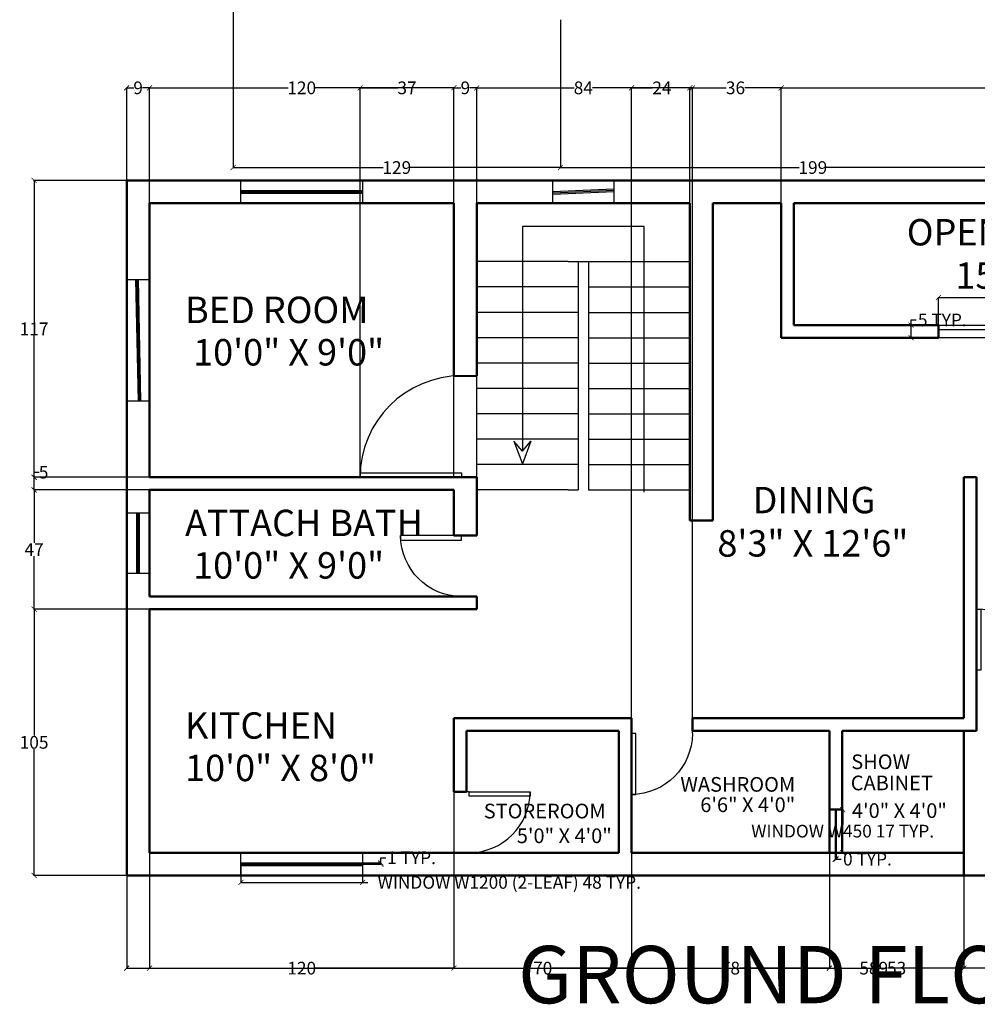
# Model space of a CAD drawing. Units: inches. Extents: x 1455 to 5994, y -182 to 2370.
# Tile 1 of 8: x 1509 to 1887, y 1415 to 1803. Entities that reach past the tile are written whole.
import ezdxf

# ---------------------------------------------------------------- set-up
doc = ezdxf.new("R2010")
doc.units = ezdxf.units.IN
doc.header["$MEASUREMENT"] = 0
for name, color, linetype, lineweight in [('A-ANNO-DIMS', 2, 'Continuous', 18), ('A-ANNO-TEXT', 7, 'Continuous', 25), ('A-AREA-IDEN', 7, 'Continuous', 18), ('A-DOOR', 5, 'Continuous', 25), ('A-FLOR-STRS', 3, 'Continuous', 25), ('A-GLAZ', 4, 'Continuous', 25), ('A-WALL', 7, 'Continuous', 50)]:
    doc.layers.add(name, color=color, linetype=linetype, lineweight=lineweight)
doc.styles.get("Standard").update_dxf_attribs({"font": 'arial.ttf'})
doc.dimstyles.get("Standard").update_dxf_attribs({"dimtxt": 5, "dimasz": 2, "dimexe": 0.18, "dimexo": 0.0625, "dimgap": 0.09, "dimtad": 0, "dimtih": 1, "dimtoh": 1, "dimdec": 1, "dimzin": 0, "dimdsep": 46, "dimlunit": 3, "dimtxsty": 'Standard', "dimblk": 'ARCHTICK', "dimcen": 0.09, "dimadec": 0, "dimazin": 0, "dimtfac": 1, "dimtdec": 1, "dimtofl": 0, "dimtmove": 0, "dimatfit": 3, "dimfxl": 1, "dimtolj": 1, "dimtzin": 0, "dimarcsym": 0})

# ---------------------------------------------------------------- blocks, each defined once
blk = doc.blocks.new('*U3')
for p, q in [((0, 0), (0, -6)), ((24, 0), (24, -6))]:
    blk.add_line(p, q)
blk.add_lwpolyline([(0, 0), (0, 24), (1.75, 24), (1.75, 0)], close=True)
blk.add_arc((0, 0), 24, 0, 90)
blk = doc.blocks.new('*U4')
for p, q in [((0, 0), (0, -6)), ((40, 0), (40, -6))]:
    blk.add_line(p, q)
blk.add_lwpolyline([(0, 0), (0, 40), (1.75, 40), (1.75, 0)], close=True)
blk.add_arc((0, 0), 40, 0, 90)
blk = doc.blocks.new('DOOR-SLIDING')
for p, q in [((37.51, 2.96), (37.51, 4.69)), ((0, 2.96), (37.51, 2.96)), ((34.07, 1.25), (34.07, 2.97)), ((72, 1.25), (34.07, 1.25)), ((37.51, 2.96), (72, 2.96))]:
    blk.add_line(p, q)
blk.add_lwpolyline([(0, 4.69), (72, 4.69), (72, -0.31), (0, -0.31)], close=True)
blk = doc.blocks.new('WIN-600')
for p, q in [((0, 0), (0, 24)), ((0.5, 0), (0.5, 24)), ((1, 0), (1, 24))]:
    blk.add_line(p, q)
blk = doc.blocks.new('WIN-1200')
for p, q in [((0, 1), (48, 1)), ((0, 0.5), (48, 0.5)), ((0, 0), (48, 0))]:
    blk.add_line(p, q)
blk = doc.blocks.new('WIN-1200-2L')
for p, q in [((0, 0.5), (48, 0.5)), ((0, 0), (48, 0))]:
    blk.add_line(p, q)
blk = doc.blocks.new('WIN-450')
for p, q in [((0, 17), (0, 0)), ((0.2, 17), (0.2, 0)), ((0.4, 17), (0.4, 0))]:
    blk.add_line(p, q)
blk = doc.blocks.new('_ArchTick')
at = {"color": 0, "linetype": 'ByBlock', "const_width": 0.15}
blk.add_lwpolyline([(-0.5, -0.5), (0.5, 0.5)], dxfattribs=at)
blk = doc.blocks.new('*D25')
at = {"layer": 'A-ANNO-DIMS', "color": 0, "lineweight": -2, "transparency": 16777216}
for p, q in [((1596.31, 1470.12), (1596.31, 1462.81)), ((1644.31, 1470.12), (1644.31, 1462.81)), ((1596.31, 1462.99), (1644.31, 1462.99)), ((1644.31, 1462.99), (1646.31, 1462.99))]:
    blk.add_line(p, q, dxfattribs=at)
at = {"layer": 'Defpoints', "color": 0, "lineweight": 25, "transparency": 16777216}
for p in [(1596.31, 1470.19), (1644.31, 1470.19), (1644.31, 1462.99)]:
    blk.add_point(p, dxfattribs=at)
at = {"layer": 'A-ANNO-DIMS', "color": 0, "lineweight": -2, "transparency": 16777216, "xscale": 2, "yscale": 2, "zscale": 2, "rotation": 180}
blk.add_blockref('_ArchTick', (1596.31, 1462.99), dxfattribs=at)
at = {"layer": 'A-ANNO-DIMS', "color": 0, "lineweight": -2, "transparency": 16777216, "xscale": 2, "yscale": 2, "zscale": 2}
blk.add_blockref('_ArchTick', (1644.31, 1462.99), dxfattribs=at)
at = {"layer": 'A-ANNO-DIMS', "color": 0, "transparency": 16777216, "insert": (1702.14, 1462.99), "char_height": 5, "attachment_point": 5}
blk.add_mtext('\\A1;WINDOW W1200 (2-LEAF) 48 TYP.', dxfattribs=at)
blk = doc.blocks.new('*D26')
at = {"layer": 'A-ANNO-DIMS', "color": 0, "lineweight": -2, "transparency": 16777216}
for p, q in [((1651.51, 1470.69), (1651.51, 1472.69)), ((1651.51, 1472.69), (1653.51, 1472.69)), ((1644.37, 1470.69), (1651.69, 1470.69)), ((1644.37, 1470.19), (1651.69, 1470.19)), ((1651.51, 1470.19), (1651.51, 1470.69))]:
    blk.add_line(p, q, dxfattribs=at)
at = {"layer": 'Defpoints', "color": 0, "lineweight": 25, "transparency": 16777216}
for p in [(1644.31, 1470.69), (1644.31, 1470.19), (1651.51, 1470.69)]:
    blk.add_point(p, dxfattribs=at)
at = {"layer": 'A-ANNO-DIMS', "color": 0, "lineweight": -2, "transparency": 16777216, "xscale": 2, "yscale": 2, "zscale": 2}
for p, rotation in [((1651.51, 1470.69), 90), ((1651.51, 1470.19), 270)]:
    blk.add_blockref('_ArchTick', p, dxfattribs=dict(at, rotation=rotation))
at = {"layer": 'A-ANNO-DIMS', "color": 0, "transparency": 16777216, "insert": (1663.59, 1472.69), "char_height": 5, "attachment_point": 5}
blk.add_mtext('\\A1;1 TYP.', dxfattribs=at)
blk = doc.blocks.new('*D27')
at = {"layer": 'A-ANNO-DIMS', "color": 0, "lineweight": -2, "transparency": 16777216}
for p, q in [((1831.07, 1491.69), (1833.74, 1491.69)), ((1833.56, 1491.69), (1833.56, 1485.86)), ((1833.56, 1474.69), (1833.56, 1480.51)), ((1831.07, 1474.69), (1833.74, 1474.69))]:
    blk.add_line(p, q, dxfattribs=at)
at = {"layer": 'Defpoints', "color": 0, "lineweight": 25, "transparency": 16777216}
for p in [(1831.01, 1491.69), (1833.56, 1491.69), (1831.01, 1474.69)]:
    blk.add_point(p, dxfattribs=at)
at = {"layer": 'A-ANNO-DIMS', "color": 0, "lineweight": -2, "transparency": 16777216, "xscale": 2, "yscale": 2, "zscale": 2}
for p, rotation in [((1833.56, 1491.69), 90), ((1833.56, 1474.69), 270)]:
    blk.add_blockref('_ArchTick', p, dxfattribs=dict(at, rotation=rotation))
at = {"layer": 'A-ANNO-DIMS', "color": 0, "transparency": 16777216, "insert": (1833.56, 1483.19), "char_height": 5, "attachment_point": 5}
blk.add_mtext('\\A1;WINDOW W450 17 TYP.', dxfattribs=at)
blk = doc.blocks.new('*D28')
at = {"layer": 'A-ANNO-DIMS', "color": 0, "lineweight": -2, "transparency": 16777216}
for p, q in [((1830.61, 1474.62), (1830.61, 1471.96)), ((1830.61, 1472.14), (1831.01, 1472.14)), ((1831.01, 1474.62), (1831.01, 1471.96)), ((1831.01, 1472.14), (1833.01, 1472.14))]:
    blk.add_line(p, q, dxfattribs=at)
at = {"layer": 'Defpoints', "color": 0, "lineweight": 25, "transparency": 16777216}
for p in [(1830.61, 1474.69), (1831.01, 1474.69), (1831.01, 1472.14)]:
    blk.add_point(p, dxfattribs=at)
at = {"layer": 'A-ANNO-DIMS', "color": 0, "lineweight": -2, "transparency": 16777216, "xscale": 2, "yscale": 2, "zscale": 2, "rotation": 180}
blk.add_blockref('_ArchTick', (1830.61, 1472.14), dxfattribs=at)
at = {"layer": 'A-ANNO-DIMS', "color": 0, "lineweight": -2, "transparency": 16777216, "xscale": 2, "yscale": 2, "zscale": 2}
blk.add_blockref('_ArchTick', (1831.01, 1472.14), dxfattribs=at)
at = {"layer": 'A-ANNO-DIMS', "color": 0, "transparency": 16777216, "insert": (1843.33, 1472.14), "char_height": 5, "attachment_point": 5}
blk.add_mtext('\\A1;0 TYP.', dxfattribs=at)
blk = doc.blocks.new('*D29')
at = {"layer": 'A-ANNO-DIMS', "color": 0, "lineweight": -2, "transparency": 16777216}
for p, q in [((1871.31, 1682.75), (1871.31, 1693.67)), ((1871.31, 1693.49), (1943.31, 1693.49)), ((1943.31, 1682.75), (1943.31, 1693.67)), ((1943.31, 1693.49), (1945.31, 1693.49))]:
    blk.add_line(p, q, dxfattribs=at)
at = {"layer": 'Defpoints', "color": 0, "lineweight": 25, "transparency": 16777216}
for p in [(1943.31, 1693.49), (1871.31, 1682.69), (1943.31, 1682.69)]:
    blk.add_point(p, dxfattribs=at)
at = {"layer": 'A-ANNO-DIMS', "color": 0, "lineweight": -2, "transparency": 16777216, "xscale": 2, "yscale": 2, "zscale": 2, "rotation": 180}
blk.add_blockref('_ArchTick', (1871.31, 1693.49), dxfattribs=at)
at = {"layer": 'A-ANNO-DIMS', "color": 0, "lineweight": -2, "transparency": 16777216, "xscale": 2, "yscale": 2, "zscale": 2}
blk.add_blockref('_ArchTick', (1943.31, 1693.49), dxfattribs=at)
at = {"layer": 'A-ANNO-DIMS', "color": 0, "transparency": 16777216, "insert": (1983.95, 1693.49), "char_height": 5, "attachment_point": 5}
blk.add_mtext('\\A1;SLIDING DOOR 72 TYP.', dxfattribs=at)
blk = doc.blocks.new('*D30')
at = {"layer": 'A-ANNO-DIMS', "color": 0, "lineweight": -2, "transparency": 16777216}
for p, q in [((1860.51, 1682.69), (1860.51, 1684.69)), ((1860.51, 1684.69), (1862.51, 1684.69)), ((1871.25, 1682.69), (1860.33, 1682.69)), ((1860.51, 1677.69), (1860.51, 1682.69)), ((1871.25, 1677.69), (1860.33, 1677.69))]:
    blk.add_line(p, q, dxfattribs=at)
at = {"layer": 'Defpoints', "color": 0, "lineweight": 25, "transparency": 16777216}
for p in [(1860.51, 1682.69), (1871.31, 1682.69), (1871.31, 1677.69)]:
    blk.add_point(p, dxfattribs=at)
at = {"layer": 'A-ANNO-DIMS', "color": 0, "lineweight": -2, "transparency": 16777216, "xscale": 2, "yscale": 2, "zscale": 2}
for p, rotation in [((1860.51, 1682.69), 90), ((1860.51, 1677.69), 270)]:
    blk.add_blockref('_ArchTick', p, dxfattribs=dict(at, rotation=rotation))
at = {"layer": 'A-ANNO-DIMS', "color": 0, "transparency": 16777216, "insert": (1872.83, 1684.69), "char_height": 5, "attachment_point": 5}
blk.add_mtext('\\A1;5 TYP.', dxfattribs=at)
blk = doc.blocks.new('*D35')
at = {"layer": 'A-ANNO-DIMS', "color": 0, "lineweight": -2, "transparency": 16777216}
for p, q in [((1593.29, 1828.67), (1593.29, 1744.59)), ((1722.29, 1802.99), (1722.29, 1744.59)), ((1593.29, 1744.77), (1652.41, 1744.77)), ((1722.29, 1744.77), (1663.18, 1744.77))]:
    blk.add_line(p, q, dxfattribs=at)
at = {"layer": 'Defpoints', "color": 0, "lineweight": 25, "transparency": 16777216}
for p in [(1593.29, 1828.73), (1722.29, 1803.05), (1722.29, 1744.77)]:
    blk.add_point(p, dxfattribs=at)
at = {"layer": 'A-ANNO-DIMS', "color": 0, "lineweight": -2, "transparency": 16777216, "xscale": 2, "yscale": 2, "zscale": 2, "rotation": 180}
blk.add_blockref('_ArchTick', (1593.29, 1744.77), dxfattribs=at)
at = {"layer": 'A-ANNO-DIMS', "color": 0, "lineweight": -2, "transparency": 16777216, "xscale": 2, "yscale": 2, "zscale": 2}
blk.add_blockref('_ArchTick', (1722.29, 1744.77), dxfattribs=at)
at = {"layer": 'A-ANNO-DIMS', "color": 0, "transparency": 16777216, "insert": (1657.79, 1744.77), "char_height": 5, "attachment_point": 5}
blk.add_mtext('\\A1;129', dxfattribs=at)
blk = doc.blocks.new('*D36')
at = {"layer": 'A-ANNO-DIMS', "color": 0, "lineweight": -2, "transparency": 16777216}
for p, q in [((1722.29, 1802.99), (1722.29, 1744.59)), ((1921.29, 1801.67), (1921.29, 1744.59)), ((1722.29, 1744.77), (1816.41, 1744.77)), ((1921.29, 1744.77), (1827.18, 1744.77))]:
    blk.add_line(p, q, dxfattribs=at)
at = {"layer": 'Defpoints', "color": 0, "lineweight": 25, "transparency": 16777216}
for p in [(1722.29, 1803.05), (1921.29, 1801.73), (1921.29, 1744.77)]:
    blk.add_point(p, dxfattribs=at)
at = {"layer": 'A-ANNO-DIMS', "color": 0, "lineweight": -2, "transparency": 16777216, "xscale": 2, "yscale": 2, "zscale": 2, "rotation": 180}
blk.add_blockref('_ArchTick', (1722.29, 1744.77), dxfattribs=at)
at = {"layer": 'A-ANNO-DIMS', "color": 0, "lineweight": -2, "transparency": 16777216, "xscale": 2, "yscale": 2, "zscale": 2}
blk.add_blockref('_ArchTick', (1921.29, 1744.77), dxfattribs=at)
at = {"layer": 'A-ANNO-DIMS', "color": 0, "transparency": 16777216, "insert": (1821.79, 1744.77), "char_height": 5, "attachment_point": 5}
blk.add_mtext('\\A1;199', dxfattribs=at)
blk = doc.blocks.new('*D43')
at = {"layer": 'A-ANNO-DIMS', "color": 0, "lineweight": -2, "transparency": 16777216}
for p, q in [((1551.31, 1465.62), (1551.31, 1429.01)), ((2140.31, 1465.62), (2140.31, 1429.01)), ((1551.31, 1429.19), (1840.19, 1429.19)), ((2140.31, 1429.19), (1851.43, 1429.19))]:
    blk.add_line(p, q, dxfattribs=at)
at = {"layer": 'Defpoints', "color": 0, "lineweight": 25, "transparency": 16777216}
for p in [(1551.31, 1465.69), (2140.31, 1465.69), (2140.31, 1429.19)]:
    blk.add_point(p, dxfattribs=at)
at = {"layer": 'A-ANNO-DIMS', "color": 0, "lineweight": -2, "transparency": 16777216, "xscale": 2, "yscale": 2, "zscale": 2, "rotation": 180}
blk.add_blockref('_ArchTick', (1551.31, 1429.19), dxfattribs=at)
at = {"layer": 'A-ANNO-DIMS', "color": 0, "lineweight": -2, "transparency": 16777216, "xscale": 2, "yscale": 2, "zscale": 2}
blk.add_blockref('_ArchTick', (2140.31, 1429.19), dxfattribs=at)
at = {"layer": 'A-ANNO-DIMS', "color": 0, "transparency": 16777216, "insert": (1845.81, 1429.19), "char_height": 5, "attachment_point": 5}
blk.add_mtext('\\A1;589', dxfattribs=at)
blk = doc.blocks.new('*D45')
at = {"layer": 'A-ANNO-DIMS', "color": 0, "lineweight": -2, "transparency": 16777216}
for p, q in [((1551.31, 1739.75), (1551.31, 1776.37)), ((1551.31, 1776.19), (1554.08, 1776.19)), ((1560.31, 1776.19), (1557.55, 1776.19)), ((1560.31, 1700.75), (1560.31, 1776.37))]:
    blk.add_line(p, q, dxfattribs=at)
at = {"layer": 'Defpoints', "color": 0, "lineweight": 25, "transparency": 16777216}
for p in [(1560.31, 1776.19), (1551.31, 1739.69), (1560.31, 1700.69)]:
    blk.add_point(p, dxfattribs=at)
at = {"layer": 'A-ANNO-DIMS', "color": 0, "lineweight": -2, "transparency": 16777216, "xscale": 2, "yscale": 2, "zscale": 2, "rotation": 180}
blk.add_blockref('_ArchTick', (1551.31, 1776.19), dxfattribs=at)
at = {"layer": 'A-ANNO-DIMS', "color": 0, "lineweight": -2, "transparency": 16777216, "xscale": 2, "yscale": 2, "zscale": 2}
blk.add_blockref('_ArchTick', (1560.31, 1776.19), dxfattribs=at)
at = {"layer": 'A-ANNO-DIMS', "color": 0, "transparency": 16777216, "insert": (1555.81, 1776.19), "char_height": 5, "attachment_point": 5}
blk.add_mtext('\\A1;9', dxfattribs=at)
blk = doc.blocks.new('*D46')
at = {"layer": 'A-ANNO-DIMS', "color": 0, "lineweight": -2, "transparency": 16777216}
for p, q in [((1560.31, 1700.75), (1560.31, 1776.37)), ((1560.31, 1776.19), (1614.94, 1776.19)), ((1680.31, 1776.19), (1625.68, 1776.19)), ((1680.31, 1730.75), (1680.31, 1776.37))]:
    blk.add_line(p, q, dxfattribs=at)
at = {"layer": 'Defpoints', "color": 0, "lineweight": 25, "transparency": 16777216}
for p in [(1680.31, 1776.19), (1680.31, 1730.69), (1560.31, 1700.69)]:
    blk.add_point(p, dxfattribs=at)
at = {"layer": 'A-ANNO-DIMS', "color": 0, "lineweight": -2, "transparency": 16777216, "xscale": 2, "yscale": 2, "zscale": 2, "rotation": 180}
blk.add_blockref('_ArchTick', (1560.31, 1776.19), dxfattribs=at)
at = {"layer": 'A-ANNO-DIMS', "color": 0, "lineweight": -2, "transparency": 16777216, "xscale": 2, "yscale": 2, "zscale": 2}
blk.add_blockref('_ArchTick', (1680.31, 1776.19), dxfattribs=at)
at = {"layer": 'A-ANNO-DIMS', "color": 0, "transparency": 16777216, "insert": (1620.31, 1776.19), "char_height": 5, "attachment_point": 5}
blk.add_mtext('\\A1;120', dxfattribs=at)
blk = doc.blocks.new('*D47')
at = {"layer": 'A-ANNO-DIMS', "color": 0, "lineweight": -2, "transparency": 16777216}
for p, q in [((1680.31, 1730.75), (1680.31, 1776.37)), ((1680.31, 1776.19), (1683.08, 1776.19)), ((1689.31, 1776.19), (1686.55, 1776.19)), ((1689.31, 1730.75), (1689.31, 1776.37))]:
    blk.add_line(p, q, dxfattribs=at)
at = {"layer": 'Defpoints', "color": 0, "lineweight": 25, "transparency": 16777216}
for p in [(1689.31, 1776.19), (1680.31, 1730.69), (1689.31, 1730.69)]:
    blk.add_point(p, dxfattribs=at)
at = {"layer": 'A-ANNO-DIMS', "color": 0, "lineweight": -2, "transparency": 16777216, "xscale": 2, "yscale": 2, "zscale": 2, "rotation": 180}
blk.add_blockref('_ArchTick', (1680.31, 1776.19), dxfattribs=at)
at = {"layer": 'A-ANNO-DIMS', "color": 0, "lineweight": -2, "transparency": 16777216, "xscale": 2, "yscale": 2, "zscale": 2}
blk.add_blockref('_ArchTick', (1689.31, 1776.19), dxfattribs=at)
at = {"layer": 'A-ANNO-DIMS', "color": 0, "transparency": 16777216, "insert": (1684.81, 1776.19), "char_height": 5, "attachment_point": 5}
blk.add_mtext('\\A1;9', dxfattribs=at)
blk = doc.blocks.new('*D48')
at = {"layer": 'A-ANNO-DIMS', "color": 0, "lineweight": -2, "transparency": 16777216}
for p, q in [((1689.31, 1730.75), (1689.31, 1776.37)), ((1689.31, 1776.19), (1727.65, 1776.19)), ((1773.31, 1776.19), (1734.98, 1776.19)), ((1773.31, 1730.75), (1773.31, 1776.37))]:
    blk.add_line(p, q, dxfattribs=at)
at = {"layer": 'Defpoints', "color": 0, "lineweight": 25, "transparency": 16777216}
for p in [(1773.31, 1776.19), (1689.31, 1730.69), (1773.31, 1730.69)]:
    blk.add_point(p, dxfattribs=at)
at = {"layer": 'A-ANNO-DIMS', "color": 0, "lineweight": -2, "transparency": 16777216, "xscale": 2, "yscale": 2, "zscale": 2, "rotation": 180}
blk.add_blockref('_ArchTick', (1689.31, 1776.19), dxfattribs=at)
at = {"layer": 'A-ANNO-DIMS', "color": 0, "lineweight": -2, "transparency": 16777216, "xscale": 2, "yscale": 2, "zscale": 2}
blk.add_blockref('_ArchTick', (1773.31, 1776.19), dxfattribs=at)
at = {"layer": 'A-ANNO-DIMS', "color": 0, "transparency": 16777216, "insert": (1731.31, 1776.19), "char_height": 5, "attachment_point": 5}
blk.add_mtext('\\A1;84', dxfattribs=at)
blk = doc.blocks.new('*D49')
at = {"layer": 'A-ANNO-DIMS', "color": 0, "lineweight": -2, "transparency": 16777216}
for p, q in [((1773.31, 1730.75), (1773.31, 1776.37)), ((1773.31, 1776.19), (1787.64, 1776.19)), ((1809.31, 1776.19), (1794.98, 1776.19)), ((1809.31, 1730.75), (1809.31, 1776.37))]:
    blk.add_line(p, q, dxfattribs=at)
at = {"layer": 'Defpoints', "color": 0, "lineweight": 25, "transparency": 16777216}
for p in [(1809.31, 1776.19), (1773.31, 1730.69), (1809.31, 1730.69)]:
    blk.add_point(p, dxfattribs=at)
at = {"layer": 'A-ANNO-DIMS', "color": 0, "lineweight": -2, "transparency": 16777216, "xscale": 2, "yscale": 2, "zscale": 2, "rotation": 180}
blk.add_blockref('_ArchTick', (1773.31, 1776.19), dxfattribs=at)
at = {"layer": 'A-ANNO-DIMS', "color": 0, "lineweight": -2, "transparency": 16777216, "xscale": 2, "yscale": 2, "zscale": 2}
blk.add_blockref('_ArchTick', (1809.31, 1776.19), dxfattribs=at)
at = {"layer": 'A-ANNO-DIMS', "color": 0, "transparency": 16777216, "insert": (1791.31, 1776.19), "char_height": 5, "attachment_point": 5}
blk.add_mtext('\\A1;36', dxfattribs=at)
blk = doc.blocks.new('*D50')
at = {"layer": 'A-ANNO-DIMS', "color": 0, "lineweight": -2, "transparency": 16777216}
for p, q in [((1809.31, 1730.75), (1809.31, 1776.37)), ((1809.31, 1776.19), (1901.94, 1776.19)), ((2005.31, 1776.19), (1912.69, 1776.19)), ((2005.31, 1730.75), (2005.31, 1776.37))]:
    blk.add_line(p, q, dxfattribs=at)
at = {"layer": 'Defpoints', "color": 0, "lineweight": 25, "transparency": 16777216}
for p in [(2005.31, 1776.19), (1809.31, 1730.69), (2005.31, 1730.69)]:
    blk.add_point(p, dxfattribs=at)
at = {"layer": 'A-ANNO-DIMS', "color": 0, "lineweight": -2, "transparency": 16777216, "xscale": 2, "yscale": 2, "zscale": 2, "rotation": 180}
blk.add_blockref('_ArchTick', (1809.31, 1776.19), dxfattribs=at)
at = {"layer": 'A-ANNO-DIMS', "color": 0, "lineweight": -2, "transparency": 16777216, "xscale": 2, "yscale": 2, "zscale": 2}
blk.add_blockref('_ArchTick', (2005.31, 1776.19), dxfattribs=at)
at = {"layer": 'A-ANNO-DIMS', "color": 0, "transparency": 16777216, "insert": (1907.31, 1776.19), "char_height": 5, "attachment_point": 5}
blk.add_mtext('\\A1;196', dxfattribs=at)
blk = doc.blocks.new('*D53')
at = {"layer": 'A-ANNO-DIMS', "color": 0, "lineweight": -2, "transparency": 16777216}
for p, q in [((1560.25, 1570.69), (1514.63, 1570.69)), ((1514.81, 1570.69), (1514.81, 1520.83)), ((1514.81, 1465.69), (1514.81, 1515.54)), ((2140.25, 1465.69), (1514.63, 1465.69))]:
    blk.add_line(p, q, dxfattribs=at)
at = {"layer": 'Defpoints', "color": 0, "lineweight": 25, "transparency": 16777216}
for p in [(1514.81, 1570.69), (1560.31, 1570.69), (2140.31, 1465.69)]:
    blk.add_point(p, dxfattribs=at)
at = {"layer": 'A-ANNO-DIMS', "color": 0, "lineweight": -2, "transparency": 16777216, "xscale": 2, "yscale": 2, "zscale": 2}
for p, rotation in [((1514.81, 1570.69), 90), ((1514.81, 1465.69), 270)]:
    blk.add_blockref('_ArchTick', p, dxfattribs=dict(at, rotation=rotation))
at = {"layer": 'A-ANNO-DIMS', "color": 0, "transparency": 16777216, "insert": (1514.81, 1518.19), "char_height": 5, "attachment_point": 5}
blk.add_mtext('\\A1;105', dxfattribs=at)
blk = doc.blocks.new('*D54')
at = {"layer": 'A-ANNO-DIMS', "color": 0, "lineweight": -2, "transparency": 16777216}
for p, q in [((1560.249038, 1617.686089), (1514.631538, 1617.686089)), ((1514.811538, 1617.686089), (1514.811538, 1596.776089)), ((1514.811538, 1570.686089), (1514.811538, 1591.596089)), ((1560.249038, 1570.686089), (1514.631538, 1570.686089))]:
    blk.add_line(p, q, dxfattribs=at)
at = {"layer": 'Defpoints', "color": 0, "lineweight": 25, "transparency": 16777216}
for p in [(1514.811538, 1617.686089), (1560.311538, 1617.686089), (1560.311538, 1570.686089)]:
    blk.add_point(p, dxfattribs=at)
at = {"layer": 'A-ANNO-DIMS', "color": 0, "lineweight": -2, "transparency": 16777216, "xscale": 2, "yscale": 2, "zscale": 2}
for p, rotation in [((1514.811538, 1617.686089), 90), ((1514.811538, 1570.686089), 270)]:
    blk.add_blockref('_ArchTick', p, dxfattribs=dict(at, rotation=rotation))
at = {"layer": 'A-ANNO-DIMS', "color": 0, "transparency": 16777216, "insert": (1514.811538, 1594.186089), "char_height": 5, "attachment_point": 5}
blk.add_mtext('\\A1;47', dxfattribs=at)
blk = doc.blocks.new('*D55')
at = {"layer": 'A-ANNO-DIMS', "color": 0, "lineweight": -2, "transparency": 16777216}
for p, q in [((1560.25, 1622.69), (1514.63, 1622.69)), ((1514.81, 1622.69), (1514.81, 1624.69)), ((1514.81, 1624.69), (1516.81, 1624.69)), ((1514.81, 1617.69), (1514.81, 1622.69)), ((1560.25, 1617.69), (1514.63, 1617.69))]:
    blk.add_line(p, q, dxfattribs=at)
at = {"layer": 'Defpoints', "color": 0, "lineweight": 25, "transparency": 16777216}
for p in [(1514.81, 1622.69), (1560.31, 1622.69), (1560.31, 1617.69)]:
    blk.add_point(p, dxfattribs=at)
at = {"layer": 'A-ANNO-DIMS', "color": 0, "lineweight": -2, "transparency": 16777216, "xscale": 2, "yscale": 2, "zscale": 2}
for p, rotation in [((1514.81, 1622.69), 90), ((1514.81, 1617.69), 270)]:
    blk.add_blockref('_ArchTick', p, dxfattribs=dict(at, rotation=rotation))
at = {"layer": 'A-ANNO-DIMS', "color": 0, "transparency": 16777216, "insert": (1518.56, 1624.69), "char_height": 5, "attachment_point": 5}
blk.add_mtext('\\A1;5', dxfattribs=at)
blk = doc.blocks.new('*D56')
at = {"layer": 'A-ANNO-DIMS', "color": 0, "lineweight": -2, "transparency": 16777216}
for p, q in [((1551.25, 1739.69), (1514.63, 1739.69)), ((1514.81, 1739.69), (1514.81, 1683.79)), ((1514.81, 1622.69), (1514.81, 1678.59)), ((1560.25, 1622.69), (1514.63, 1622.69))]:
    blk.add_line(p, q, dxfattribs=at)
at = {"layer": 'Defpoints', "color": 0, "lineweight": 25, "transparency": 16777216}
for p in [(1514.81, 1739.69), (1551.31, 1739.69), (1560.31, 1622.69)]:
    blk.add_point(p, dxfattribs=at)
at = {"layer": 'A-ANNO-DIMS', "color": 0, "lineweight": -2, "transparency": 16777216, "xscale": 2, "yscale": 2, "zscale": 2}
for p, rotation in [((1514.81, 1739.69), 90), ((1514.81, 1622.69), 270)]:
    blk.add_blockref('_ArchTick', p, dxfattribs=dict(at, rotation=rotation))
at = {"layer": 'A-ANNO-DIMS', "color": 0, "transparency": 16777216, "insert": (1514.81, 1681.19), "char_height": 5, "attachment_point": 5}
blk.add_mtext('\\A1;117', dxfattribs=at)
blk = doc.blocks.new('*D60')
at = {"layer": 'A-ANNO-DIMS', "color": 0, "lineweight": -2, "transparency": 16777216}
for p, q in [((1643.31, 1622.75), (1643.31, 1776.37)), ((1643.31, 1776.19), (1658.14, 1776.19)), ((1680.31, 1776.19), (1665.48, 1776.19)), ((1680.31, 1622.75), (1680.31, 1776.37))]:
    blk.add_line(p, q, dxfattribs=at)
at = {"layer": 'Defpoints', "color": 0, "lineweight": 25, "transparency": 16777216}
for p in [(1680.31, 1776.19), (1643.31, 1622.69), (1680.31, 1622.69)]:
    blk.add_point(p, dxfattribs=at)
at = {"layer": 'A-ANNO-DIMS', "color": 0, "lineweight": -2, "transparency": 16777216, "xscale": 2, "yscale": 2, "zscale": 2, "rotation": 180}
blk.add_blockref('_ArchTick', (1643.31, 1776.19), dxfattribs=at)
at = {"layer": 'A-ANNO-DIMS', "color": 0, "lineweight": -2, "transparency": 16777216, "xscale": 2, "yscale": 2, "zscale": 2}
blk.add_blockref('_ArchTick', (1680.31, 1776.19), dxfattribs=at)
at = {"layer": 'A-ANNO-DIMS', "color": 0, "transparency": 16777216, "insert": (1661.81, 1776.19), "char_height": 5, "attachment_point": 5}
blk.add_mtext('\\A1;37', dxfattribs=at)
blk = doc.blocks.new('*D63')
at = {"layer": 'A-ANNO-DIMS', "color": 0, "lineweight": -2, "transparency": 16777216}
for p, q in [((1680.31, 1498.62), (1680.31, 1429.01)), ((1560.31, 1474.62), (1560.31, 1429.01)), ((1560.31, 1429.19), (1614.94, 1429.19)), ((1680.31, 1429.19), (1625.68, 1429.19))]:
    blk.add_line(p, q, dxfattribs=at)
at = {"layer": 'Defpoints', "color": 0, "lineweight": 25, "transparency": 16777216}
for p in [(1680.31, 1498.69), (1560.31, 1474.69), (1680.31, 1429.19)]:
    blk.add_point(p, dxfattribs=at)
at = {"layer": 'A-ANNO-DIMS', "color": 0, "lineweight": -2, "transparency": 16777216, "xscale": 2, "yscale": 2, "zscale": 2, "rotation": 180}
blk.add_blockref('_ArchTick', (1560.31, 1429.19), dxfattribs=at)
at = {"layer": 'A-ANNO-DIMS', "color": 0, "lineweight": -2, "transparency": 16777216, "xscale": 2, "yscale": 2, "zscale": 2}
blk.add_blockref('_ArchTick', (1680.31, 1429.19), dxfattribs=at)
at = {"layer": 'A-ANNO-DIMS', "color": 0, "transparency": 16777216, "insert": (1620.31, 1429.19), "char_height": 5, "attachment_point": 5}
blk.add_mtext('\\A1;120', dxfattribs=at)
blk = doc.blocks.new('*D64')
at = {"layer": 'A-ANNO-DIMS', "color": 0, "lineweight": -2, "transparency": 16777216}
for p, q in [((1680.31, 1498.62), (1680.31, 1429.01)), ((1750.31, 1474.62), (1750.31, 1429.01)), ((1680.31, 1429.19), (1711.67, 1429.19)), ((1750.31, 1429.19), (1718.95, 1429.19))]:
    blk.add_line(p, q, dxfattribs=at)
at = {"layer": 'Defpoints', "color": 0, "lineweight": 25, "transparency": 16777216}
for p in [(1680.31, 1498.69), (1750.31, 1474.69), (1750.31, 1429.19)]:
    blk.add_point(p, dxfattribs=at)
at = {"layer": 'A-ANNO-DIMS', "color": 0, "lineweight": -2, "transparency": 16777216, "xscale": 2, "yscale": 2, "zscale": 2, "rotation": 180}
blk.add_blockref('_ArchTick', (1680.31, 1429.19), dxfattribs=at)
at = {"layer": 'A-ANNO-DIMS', "color": 0, "lineweight": -2, "transparency": 16777216, "xscale": 2, "yscale": 2, "zscale": 2}
blk.add_blockref('_ArchTick', (1750.31, 1429.19), dxfattribs=at)
at = {"layer": 'A-ANNO-DIMS', "color": 0, "transparency": 16777216, "insert": (1715.31, 1429.19), "char_height": 5, "attachment_point": 5}
blk.add_mtext('\\A1;70', dxfattribs=at)
blk = doc.blocks.new('*D65')
at = {"layer": 'A-ANNO-DIMS', "color": 0, "lineweight": -2, "transparency": 16777216}
for p, q in [((1750.31, 1474.62), (1750.31, 1429.01)), ((1828.31, 1474.62), (1828.31, 1429.01)), ((1750.31, 1429.19), (1785.66, 1429.19)), ((1828.31, 1429.19), (1792.97, 1429.19))]:
    blk.add_line(p, q, dxfattribs=at)
at = {"layer": 'Defpoints', "color": 0, "lineweight": 25, "transparency": 16777216}
for p in [(1750.31, 1474.69), (1828.31, 1474.69), (1828.31, 1429.19)]:
    blk.add_point(p, dxfattribs=at)
at = {"layer": 'A-ANNO-DIMS', "color": 0, "lineweight": -2, "transparency": 16777216, "xscale": 2, "yscale": 2, "zscale": 2, "rotation": 180}
blk.add_blockref('_ArchTick', (1750.31, 1429.19), dxfattribs=at)
at = {"layer": 'A-ANNO-DIMS', "color": 0, "lineweight": -2, "transparency": 16777216, "xscale": 2, "yscale": 2, "zscale": 2}
blk.add_blockref('_ArchTick', (1828.31, 1429.19), dxfattribs=at)
at = {"layer": 'A-ANNO-DIMS', "color": 0, "transparency": 16777216, "insert": (1789.31, 1429.19), "char_height": 5, "attachment_point": 5}
blk.add_mtext('\\A1;78', dxfattribs=at)
blk = doc.blocks.new('*D66')
at = {"layer": 'A-ANNO-DIMS', "color": 0, "lineweight": -2, "transparency": 16777216}
for p, q in [((1828.31, 1474.62), (1828.31, 1429.01)), ((1881.31, 1474.62), (1881.31, 1429.01)), ((1828.31, 1429.19), (1851.14, 1429.19)), ((1881.31, 1429.19), (1858.48, 1429.19))]:
    blk.add_line(p, q, dxfattribs=at)
at = {"layer": 'Defpoints', "color": 0, "lineweight": 25, "transparency": 16777216}
for p in [(1828.31, 1474.69), (1881.31, 1474.69), (1881.31, 1429.19)]:
    blk.add_point(p, dxfattribs=at)
at = {"layer": 'A-ANNO-DIMS', "color": 0, "lineweight": -2, "transparency": 16777216, "xscale": 2, "yscale": 2, "zscale": 2, "rotation": 180}
blk.add_blockref('_ArchTick', (1828.31, 1429.19), dxfattribs=at)
at = {"layer": 'A-ANNO-DIMS', "color": 0, "lineweight": -2, "transparency": 16777216, "xscale": 2, "yscale": 2, "zscale": 2}
blk.add_blockref('_ArchTick', (1881.31, 1429.19), dxfattribs=at)
at = {"layer": 'A-ANNO-DIMS', "color": 0, "transparency": 16777216, "insert": (1854.81, 1429.19), "char_height": 5, "attachment_point": 5}
blk.add_mtext('\\A1;53', dxfattribs=at)
blk = doc.blocks.new('*D67')
at = {"layer": 'A-ANNO-DIMS', "color": 0, "lineweight": -2, "transparency": 16777216}
for p, q in [((1750.31, 1527.75), (1750.31, 1776.37)), ((1750.31, 1776.19), (1758.61, 1776.19)), ((1774.31, 1776.19), (1766.02, 1776.19)), ((1774.31, 1527.75), (1774.31, 1776.37))]:
    blk.add_line(p, q, dxfattribs=at)
at = {"layer": 'Defpoints', "color": 0, "lineweight": 25, "transparency": 16777216}
for p in [(1774.31, 1776.19), (1750.31, 1527.69), (1774.31, 1527.69)]:
    blk.add_point(p, dxfattribs=at)
at = {"layer": 'A-ANNO-DIMS', "color": 0, "lineweight": -2, "transparency": 16777216, "xscale": 2, "yscale": 2, "zscale": 2, "rotation": 180}
blk.add_blockref('_ArchTick', (1750.31, 1776.19), dxfattribs=at)
at = {"layer": 'A-ANNO-DIMS', "color": 0, "lineweight": -2, "transparency": 16777216, "xscale": 2, "yscale": 2, "zscale": 2}
blk.add_blockref('_ArchTick', (1774.31, 1776.19), dxfattribs=at)
at = {"layer": 'A-ANNO-DIMS', "color": 0, "transparency": 16777216, "insert": (1762.31, 1776.19), "char_height": 5, "attachment_point": 5}
blk.add_mtext('\\A1;24', dxfattribs=at)

msp = doc.modelspace()

# ---------------------------------------------------------------- linework, layer by layer
at = {"layer": 'A-FLOR-STRS'}
for p, q in [((1755.3115, 1721.5573), (1707.3115, 1721.5573)), ((1707.3115, 1721.5573), (1707.3115, 1632.9997)), ((1755.3115, 1616.8618), (1755.3115, 1721.5573)), ((1725.3115, 1707.6861), (1689.3115, 1707.6861)), ((1725.3115, 1707.6861), (1737.3115, 1707.6861)), ((1729.3115, 1707.6861), (1729.3115, 1617.6861)), ((1733.3115, 1707.6861), (1733.3115, 1617.6861)), ((1737.3115, 1707.6861), (1773.3115, 1707.6861)), ((1729.3115, 1697.6861), (1689.3115, 1697.6861)), ((1733.3115, 1697.6861), (1773.3115, 1697.6861)), ((1729.3115, 1687.6861), (1689.3115, 1687.6861)), ((1733.3115, 1687.6861), (1773.3115, 1687.6861)), ((1729.3115, 1677.6861), (1689.3115, 1677.6861)), ((1733.3115, 1677.6861), (1773.3115, 1677.6861)), ((1729.3115, 1667.6861), (1689.3115, 1667.6861)), ((1733.3115, 1667.6861), (1773.3115, 1667.6861)), ((1689.3115, 1617.6861), (1689.3115, 1664.6861)), ((1729.3115, 1657.6861), (1689.3115, 1657.6861)), ((1733.3115, 1657.6861), (1773.3115, 1657.6861)), ((1729.3115, 1647.6861), (1689.3115, 1647.6861)), ((1733.3115, 1647.6861), (1773.3115, 1647.6861)), ((1729.3115, 1637.6861), (1689.3115, 1637.6861)), ((1707.3115, 1632.9997), (1703.9639, 1636.8618)), ((1703.9639, 1636.8618), (1707.3115, 1627.9809)), ((1707.3115, 1632.9997), (1710.6592, 1636.8618)), ((1710.6592, 1636.8618), (1707.3115, 1627.9809)), ((1733.3115, 1637.6861), (1773.3115, 1637.6861)), ((1729.3115, 1627.6861), (1689.3115, 1627.6861)), ((1733.3115, 1627.6861), (1773.3115, 1627.6861)), ((1725.3115, 1617.6861), (1689.3115, 1617.6861)), ((1725.3115, 1617.6861), (1729.3115, 1617.6861)), ((1733.3115, 1617.6861), (1737.3115, 1617.6861)), ((1737.3115, 1617.6861), (1773.3115, 1617.6861))]:
    msp.add_line(p, q, dxfattribs=at)
at = {"layer": 'A-GLAZ'}
msp.add_line((1596.3115, 1469.6861), (1644.3115, 1469.6861), dxfattribs=at)
for points in [[(1596.3115, 1739.6861), (1644.3115, 1739.6861), (1644.3115, 1730.6861), (1596.3115, 1730.6861)], [(1719.3115, 1739.6861), (1743.3115, 1739.6861), (1743.3115, 1730.6861), (1719.3115, 1730.6861)], [(1560.3115, 1700.6861), (1560.3115, 1652.6861), (1551.3115, 1652.6861), (1551.3115, 1700.6861)], [(1551.3115, 1584.6861), (1551.3115, 1608.6861), (1560.3115, 1608.6861), (1560.3115, 1584.6861)], [(1833.3115, 1474.6861), (1828.3115, 1474.6861), (1828.3115, 1491.6861), (1833.3115, 1491.6861)], [(1596.3115, 1474.6861), (1644.3115, 1474.6861), (1644.3115, 1465.6861), (1596.3115, 1465.6861)]]:
    msp.add_lwpolyline(points, close=True, dxfattribs=at)
at = {"layer": 'A-WALL'}
for p, q in [((1551.3115, 1739.6861), (1551.3115, 1465.6861)), ((1551.3115, 1739.6861), (2140.3115, 1739.6861)), ((1560.3115, 1730.6861), (1560.3115, 1622.6861)), ((1560.3115, 1730.6861), (1680.3115, 1730.6861)), ((1680.3115, 1730.6861), (1680.3115, 1662.5734)), ((1689.3115, 1730.6861), (1689.3115, 1662.6861)), ((1689.3115, 1730.6861), (1773.3115, 1730.6861)), ((1773.3115, 1730.6861), (1773.3115, 1605.7037)), ((1782.3115, 1730.6861), (1782.3115, 1605.7037)), ((1782.3115, 1730.6861), (1809.3115, 1730.6861)), ((1809.3115, 1730.6861), (1809.3115, 1694.6861)), ((1814.3115, 1730.6861), (2000.3115, 1730.6861)), ((1814.3115, 1730.6861), (1814.3115, 1694.6861)), ((1809.3115, 1694.6861), (1809.3115, 1677.6861)), ((1814.3115, 1694.6861), (1814.3115, 1682.6861)), ((1814.3115, 1682.6861), (1871.3115, 1682.6861)), ((1871.3115, 1682.6861), (1871.3115, 1677.6861)), ((1809.3115, 1677.6861), (1871.3115, 1677.6861)), ((1680.3115, 1662.5734), (1689.3115, 1662.6861)), ((1560.3115, 1622.6861), (1680.3115, 1622.6861)), ((1680.3115, 1622.6861), (1689.3115, 1622.6861)), ((1689.3115, 1622.6861), (1689.3115, 1617.6861)), ((1881.3115, 1622.6861), (1881.3115, 1527.6861)), ((1881.3115, 1622.6861), (1886.3115, 1622.6861)), ((1886.3115, 1622.6861), (1886.3115, 1545.6861)), ((1560.3115, 1617.6861), (1680.3115, 1617.6861)), ((1560.3115, 1617.6861), (1560.3115, 1575.6861)), ((1680.3115, 1617.6861), (1680.3115, 1599.6861)), ((1689.3115, 1617.6861), (1689.3115, 1599.6861)), ((1782.3115, 1605.7037), (1773.3115, 1605.7037)), ((1680.3115, 1599.6861), (1689.3115, 1599.6861)), ((1560.3115, 1575.6861), (1680.3115, 1575.6861)), ((1680.3115, 1575.6861), (1689.3115, 1575.6861)), ((1689.3115, 1575.6861), (1689.3115, 1570.6861)), ((1560.3115, 1570.6861), (1689.3115, 1570.6861)), ((1560.3115, 1570.6861), (1560.3115, 1474.6861)), ((1886.3115, 1545.6861), (1886.3115, 1540.6861)), ((1886.3115, 1540.6861), (1886.3115, 1522.6861)), ((1680.3115, 1527.6861), (1680.3115, 1498.6861)), ((1680.3115, 1527.6861), (1750.3115, 1527.6861)), ((1750.3115, 1522.6861), (1750.3115, 1527.6861)), ((1774.3115, 1522.6861), (1774.3115, 1527.6861)), ((1774.3115, 1527.6861), (1881.3115, 1527.6861)), ((1685.3115, 1522.6861), (1685.3115, 1498.6861)), ((1685.3115, 1522.6861), (1745.3115, 1522.6861)), ((1745.3115, 1522.6861), (1745.3115, 1474.6861)), ((1750.3115, 1522.6861), (1750.3115, 1474.6861)), ((1774.3115, 1522.6861), (1828.3115, 1522.6861)), ((1828.3115, 1522.6861), (1828.3115, 1474.6861)), ((1833.3115, 1522.6861), (1833.3115, 1474.6861)), ((1833.3115, 1522.6861), (1886.3115, 1522.6861)), ((1881.3115, 1522.6861), (1881.3115, 1465.6861)), ((1680.3115, 1498.6861), (1685.3115, 1498.6861)), ((1828.3115, 1491.6861), (1833.3115, 1491.6861)), ((1560.3115, 1474.6861), (1680.3115, 1474.6861)), ((1680.3115, 1474.6861), (1685.3115, 1474.6861)), ((1685.3115, 1474.6861), (1745.3115, 1474.6861)), ((1738.3115, 1474.6861), (1745.3115, 1474.6861)), ((1750.3115, 1474.6861), (1828.3115, 1474.6861)), ((1828.3115, 1474.6861), (1833.3115, 1474.6861)), ((1833.3115, 1474.6861), (1881.3115, 1474.6861)), ((1551.3115, 1465.6861), (2035.3115, 1465.6861))]:
    msp.add_line(p, q, dxfattribs=at)

# ---------------------------------------------------------------- block references
at = {"layer": 'A-DOOR'}
for name, p in [('DOOR-SLIDING', (1871.312, 1678)), ('*U3', (1886.3115, 1546.6861))]:
    msp.add_blockref(name, p, dxfattribs=at)
for name, p, rotation in [('*U4', (1683.3115, 1622.6861), 90.00000000000003), ('*U3', (1686.3115, 1498.6861), 270)]:
    msp.add_blockref(name, p, dxfattribs=dict(at, rotation=rotation))
at = {"layer": 'A-DOOR', "xscale": -1}
for p, rotation in [((1683.3115, 1599.6861), 90), ((1750.3115, 1521.6861), 180)]:
    msp.add_blockref('*U3', p, dxfattribs=dict(at, rotation=rotation))
at = {"layer": 'A-GLAZ'}
for name, p in [('WIN-1200', (1596.312, 1734.686)), ('WIN-600', (1555.312, 1584.686)), ('WIN-450', (1830.612, 1474.686)), ('WIN-1200-2L', (1596.312, 1470.186))]:
    msp.add_blockref(name, p, dxfattribs=at)
for name, p, rotation in [('WIN-600', (1743.322, 1735.1866), 92.3859440303877), ('WIN-1200', (1554.8117, 1700.67), 271.1934894239826)]:
    msp.add_blockref(name, p, dxfattribs=dict(at, rotation=rotation))

# ---------------------------------------------------------------- texts
at = {"layer": 'A-ANNO-TEXT'}
msp.add_text('GROUND FLOOR', height=22.629125, dxfattribs=at).set_placement((1705.5777, 1415.3353))
at = {"layer": 'A-AREA-IDEN'}
for s, height, p in [('OPEN SPACE', 10.41336, (1858.8418, 1714.0701)), ('15\'6" X 4\'0"', 10.413361, (1877.9951, 1697.0023)), ('BED ROOM ', 10.41336, (1574.3319, 1683.4665)), (' 10\'0" X 9\'0"', 10.413361, (1574.3319, 1666.7383)), ('DINING', 10.41336, (1798.0632, 1608.4878)), ('ATTACH BATH', 10.413361, (1574.3319, 1599.4712)), ('8\'3" X 12\'6"', 10.413361, (1784.1725, 1591.42)), (' 10\'0" X 9\'0"', 10.413361, (1574.3319, 1582.743)), ('KITCHEN', 10.41336, (1574.3319, 1519.6222)), ('10\'0" X 8\'0"', 10.413361, (1574.3319, 1502.894)), ('SHOW ', 5.78042, (1836.9497, 1507.6446)), ('WASHROOM', 5.78042, (1769.5717, 1498.7296)), ('CABINET', 5.78042, (1836.7434, 1499.2927)), ('6\'6" X 4\'0"', 5.780423, (1777.4317, 1490.7007)), ('4\'0" X 4\'0"', 5.780423, (1837.2104, 1488.3916)), ('STOREROOM', 5.78042, (1692.0686, 1488.2213)), ('5\'0" X 4\'0"', 5.780423, (1705.1088, 1478.4732))]:
    msp.add_text(s, height=height, dxfattribs=at).set_placement(p)

# ---------------------------------------------------------------- dimensions: what is measured, and where the dimension line sits
at = {"layer": 'A-ANNO-DIMS'}
for base, p1, p2, picture, middle in [((1722.2942, 1744.7689), (1593.2942, 1828.7288), (1722.2942, 1803.0507), '*D35', (1657.7942, 1744.7689)), ((1921.2942, 1744.7689), (1722.2942, 1803.0507), (1921.2942, 1801.7341), '*D36', (1821.7942, 1744.7689)), ((1560.3115, 1776.1861), (1551.3115, 1739.6861), (1560.3115, 1700.6861), '*D45', (1555.8115, 1776.1861)), ((1680.3115, 1776.1861), (1560.3115, 1700.6861), (1680.3115, 1730.6861), '*D46', (1620.3115, 1776.1861)), ((1680.3115, 1776.1861), (1643.3115, 1622.6861), (1680.3115, 1622.6861), '*D60', (1661.8115, 1776.1861)), ((1689.3115, 1776.1861), (1680.3115, 1730.6861), (1689.3115, 1730.6861), '*D47', (1684.8115, 1776.1861)), ((1773.3115, 1776.1861), (1689.3115, 1730.6861), (1773.3115, 1730.6861), '*D48', (1731.3115, 1776.1861)), ((1774.3115, 1776.1861), (1750.3115, 1527.6861), (1774.3115, 1527.6861), '*D67', (1762.3115, 1776.1861)), ((1809.3115, 1776.1861), (1773.3115, 1730.6861), (1809.3115, 1730.6861), '*D49', (1791.3115, 1776.1861)), ((2005.3115, 1776.1861), (1809.3115, 1730.6861), (2005.3115, 1730.6861), '*D50', (1907.3115, 1776.1861)), ((1680.3115, 1429.1861), (1560.3115, 1474.6861), (1680.3115, 1498.6861), '*D63', (1620.3115, 1429.1861)), ((1750.3115, 1429.1861), (1680.3115, 1498.6861), (1750.3115, 1474.6861), '*D64', (1715.3115, 1429.1861)), ((1828.3115, 1429.1861), (1750.3115, 1474.6861), (1828.3115, 1474.6861), '*D65', (1789.3115, 1429.1861)), ((1881.3115, 1429.1861), (1828.3115, 1474.6861), (1881.3115, 1474.6861), '*D66', (1854.8115, 1429.1861)), ((2140.3115, 1429.1861), (1551.3115, 1465.6861), (2140.3115, 1465.6861), '*D43', (1845.8115, 1429.1861))]:
    dim = msp.add_linear_dim(base=base, p1=p1, p2=p2, dimstyle='Standard', override={"dimdec": 0, "dimlfac": 1, "dimrnd": 0, "dimzin": 0, "dimdsep": 46, "dimlunit": 2}, dxfattribs=at)
    dim.commit()
    dim.dimension.update_dxf_attribs({"geometry": picture, "text_midpoint": middle})
for base, p1, p2, picture, middle in [((1514.8115, 1739.6861), (1560.3115, 1622.6861), (1551.3115, 1739.6861), '*D56', (1514.8115, 1681.1861)), ((1514.8115, 1622.6861), (1560.3115, 1617.6861), (1560.3115, 1622.6861), '*D55', (1518.5591, 1624.6861)), ((1514.8115, 1617.6861), (1560.3115, 1570.6861), (1560.3115, 1617.6861), '*D54', (1514.8115, 1594.1861)), ((1514.8115, 1570.6861), (2140.3115, 1465.6861), (1560.3115, 1570.6861), '*D53', (1514.8115, 1518.1861))]:
    dim = msp.add_linear_dim(base=base, p1=p1, p2=p2, angle=90, dimstyle='Standard', override={"dimdec": 0, "dimlfac": 1, "dimrnd": 0, "dimzin": 0, "dimdsep": 46, "dimlunit": 2}, dxfattribs=at)
    dim.commit()
    dim.dimension.update_dxf_attribs({"geometry": picture, "text_midpoint": middle})
for base, p1, p2, text, picture, middle in [((1943.3115, 1693.4861), (1871.3115, 1682.6861), (1943.3115, 1682.6861), 'SLIDING DOOR <> TYP.', '*D29', (1983.9503, 1693.4861)), ((1644.3115, 1462.9861), (1596.3115, 1470.1861), (1644.3115, 1470.1861), 'WINDOW W1200 (2-LEAF) <> TYP.', '*D25', (1702.1399, 1462.9861)), ((1831.0115, 1472.1361), (1830.6115, 1474.6861), (1831.0115, 1474.6861), '<> TYP.', '*D28', (1843.3283, 1472.1361))]:
    dim = msp.add_linear_dim(base=base, p1=p1, p2=p2, text=text, dimstyle='Standard', override={"dimdec": 0, "dimlfac": 1, "dimrnd": 0, "dimzin": 0, "dimdsep": 46, "dimlunit": 2}, dxfattribs=at)
    dim.commit()
    dim.dimension.update_dxf_attribs({"geometry": picture, "text_midpoint": middle})
for base, p1, p2, text, picture, middle in [((1860.5115, 1682.6861), (1871.3115, 1677.6861), (1871.3115, 1682.6861), '<> TYP.', '*D30', (1872.8283, 1684.6861)), ((1833.5615, 1491.6861), (1831.0115, 1474.6861), (1831.0115, 1491.6861), 'WINDOW W450 <> TYP.', '*D27', (1833.5615, 1483.1861)), ((1651.5115384547, 1470.6860889665), (1644.3115384547, 1470.1860889665), (1644.3115384547, 1470.6860889665), '<> TYP.', '*D26', (1663.5930118517, 1472.6860889665))]:
    dim = msp.add_linear_dim(base=base, p1=p1, p2=p2, angle=90, text=text, dimstyle='Standard', override={"dimdec": 0, "dimlfac": 1, "dimrnd": 0, "dimzin": 0, "dimdsep": 46, "dimlunit": 2}, dxfattribs=at)
    dim.commit()
    dim.dimension.update_dxf_attribs({"geometry": picture, "text_midpoint": middle})

doc.saveas('drawing.dxf')
